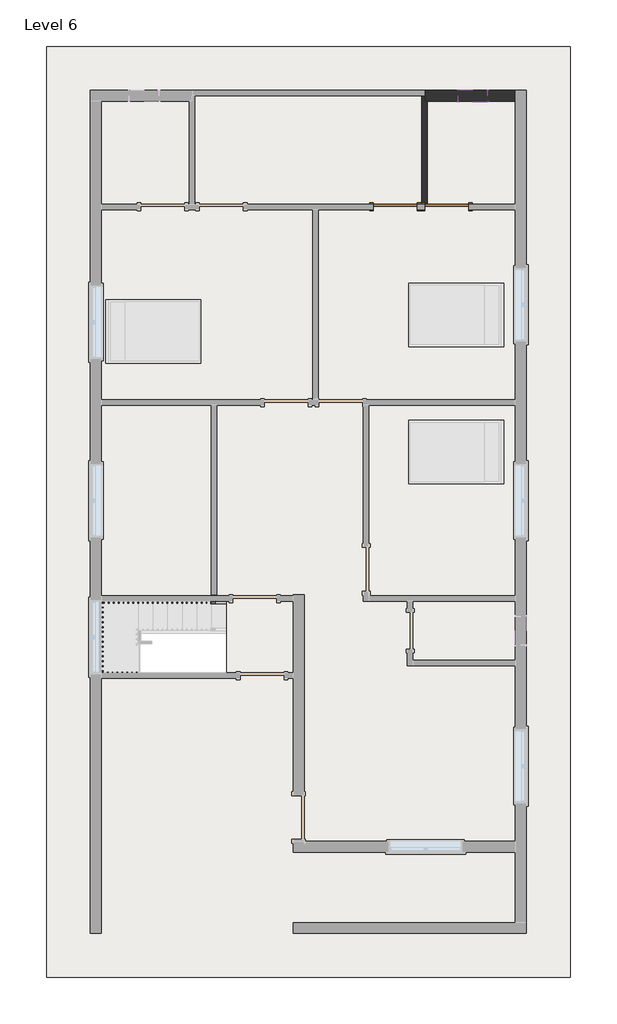
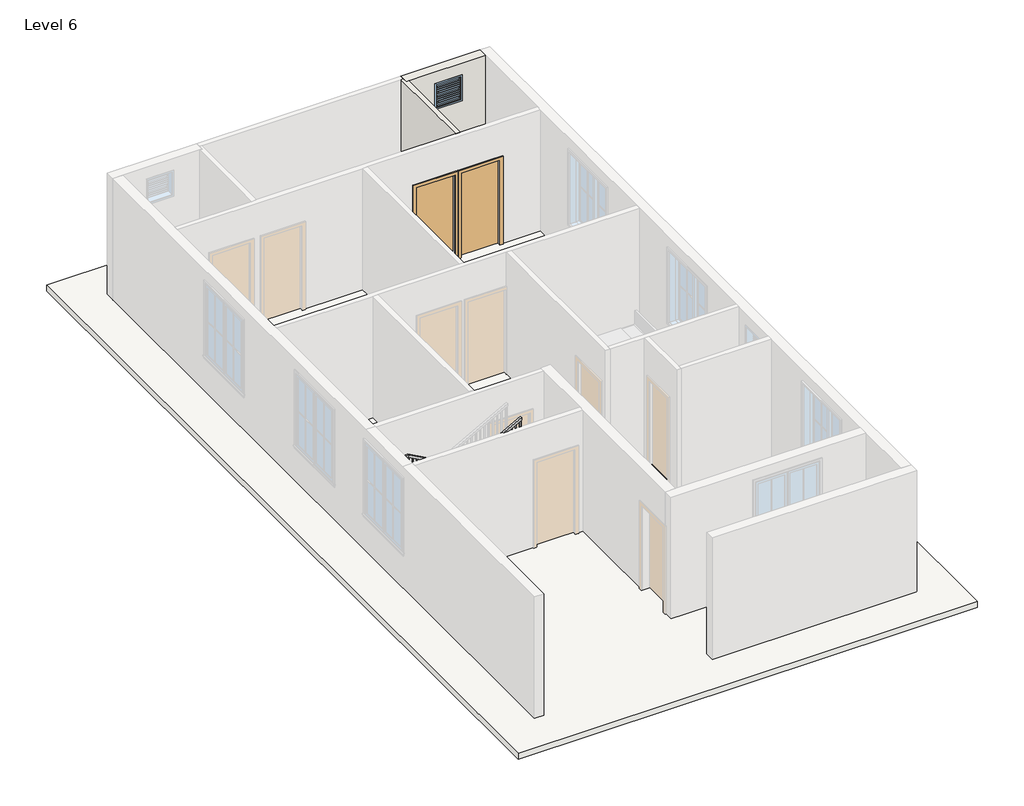
# One storey, part 2 of 3: 2 doors, 2 walls, 1 railing, 1 roof, 1 window.
"""IFC4 building model written with IfcOpenShell, lengths in millimetres."""

from ifc_helpers import new_model, si_unit, frame, origin, place, context, project, spatial, polyline, outline, extrude, faceted_brep, transform, mapped, element, save
from components import single_flush_door_3_e5f9f3c4, single_flush_door_3_305aa2a5, window_f2d8fef0

model = new_model("IFC4")

# Units and contexts
model_context = context("Model", 3, world=origin())
ifc_project = project(units=[si_unit("LENGTHUNIT", "METRE", prefix="MILLI")], contexts=[model_context])

# Site, building, storey
site = spatial("IfcSite", under=ifc_project)
building = spatial("IfcBuilding", under=site)
storey = spatial("IfcBuildingStorey", under=building, Name="Level 6", Elevation=12801.6)

# Doors
placement = place(None, origin())
single_flush_door_3_shape = single_flush_door_3_e5f9f3c4(model_context)
element("IfcDoor", 1, ObjectType="Single-Flush : DOOR 3'", at=placement, inside=storey, context=model_context, shape_type="MappedRepresentation", body=[
    mapped(single_flush_door_3_shape, transform((555.4379845, 6040.5434309, 12801.6), x_axis=(1.0, 0.0, 0.0), y_axis=(0.0, 1.0, 0.0), z_axis=(0.0, 0.0, 1.0))),
])
single_flush_door_3_2_shape = single_flush_door_3_305aa2a5(model_context)
element("IfcDoor", 2, ObjectType="Single-Flush : DOOR 3'", at=placement, inside=storey, context=model_context, shape_type="MappedRepresentation", body=[
    mapped(single_flush_door_3_2_shape, transform((1622.2379845, 6040.5434309, 12801.6), x_axis=(-1.0, 0.0, 0.0), y_axis=(0.0, -1.0, 0.0), z_axis=(0.0, 0.0, 1.0))),
])

# Railing
element("IfcRailing", 3, ObjectType="Handrail - Rectangular", at=placement, inside=storey, context=model_context, shape_type="SolidModel", body=[
    faceted_brep([(-2968.8120155, -2220.8065691, 13885.3333333), (-2968.8120155, -2220.8065691, 13827.220221), (-2968.8120155, -2170.0065691, 13827.220221), (-2968.8120155, -2170.0065691, 13885.3333333), (-4797.6120155, -2220.8065691, 14901.3333333), (-4810.7756177, -2220.8065691, 14850.5333333), (-4810.7756177, -2170.0065691, 14850.5333333), (-4797.6120155, -2170.0065691, 14901.3333333), (-5508.8120155, -2220.8065691, 14901.3333333), (-5508.8120155, -2220.8065691, 14850.5333333), (-5559.6120155, -2170.0065691, 14850.5333333), (-5559.6120155, -2170.0065691, 14901.3333333), (-5508.8120155, -3624.1565691, 14901.3333333), (-5508.8120155, -3624.1565691, 14850.5333333), (-5559.6120155, -3674.9565691, 14850.5333333), (-5559.6120155, -3674.9565691, 14901.3333333), (-5102.4120155, -3624.1565691, 14901.3333333), (-5089.2484132, -3624.1565691, 14850.5333333), (-5089.2484132, -3674.9565691, 14850.5333333), (-5102.4120155, -3674.9565691, 14901.3333333), (-2968.8120155, -3624.1565691, 16086.6666667), (-2968.8120155, -3674.9565691, 16086.6666667), (-2968.8120155, -3674.9565691, 16028.5535543), (-2968.8120155, -3624.1565691, 16028.5535543)], [[[0, 1, 2, 3]], [[1, 0, 4, 5]], [[2, 1, 5, 6]], [[3, 2, 6, 7]], [[0, 3, 7, 4]], [[5, 4, 8, 9]], [[6, 5, 9, 10]], [[7, 6, 10, 11]], [[4, 7, 11, 8]], [[9, 8, 12, 13]], [[10, 9, 13, 14]], [[11, 10, 14, 15]], [[8, 11, 15, 12]], [[13, 12, 16, 17]], [[14, 13, 17, 18]], [[15, 14, 18, 19]], [[12, 15, 19, 16]], [[20, 21, 22, 23]], [[17, 16, 20, 23]], [[18, 17, 23, 22]], [[19, 18, 22, 21]], [[16, 19, 21, 20]]]),
    extrude(outline(polyline([(16019.7341099, -2984.6870155), (16009.1507765, -3003.7370155), (15002.9333333, -3003.7370155), (15002.9333333, -2984.6870155), (16019.7341099, -2984.6870155)])), frame((0.0, -3659.0815691, 0.0), z_axis=(0.0, 1.0, 0.0), x_axis=(0.0, 0.0, 1.0)), (0.0, 0.0, 1.0), 19.05),
    extrude(outline(polyline([(15963.2896654, -3086.2870155), (15952.7063321, -3105.3370155), (15002.9333333, -3105.3370155), (15002.9333333, -3086.2870155), (15963.2896654, -3086.2870155)])), frame((0.0, -3659.0815691, 0.0), z_axis=(0.0, 1.0, 0.0), x_axis=(0.0, 0.0, 1.0)), (0.0, 0.0, 1.0), 19.05),
    extrude(outline(polyline([(15906.845221, -3187.8870155), (15896.2618876, -3206.9370155), (15002.9333333, -3206.9370155), (15002.9333333, -3187.8870155), (15906.845221, -3187.8870155)])), frame((0.0, -3659.0815691, 0.0), z_axis=(0.0, 1.0, 0.0), x_axis=(0.0, 0.0, 1.0)), (0.0, 0.0, 1.0), 19.05),
    extrude(outline(polyline([(15850.4007765, -3289.4870155), (15839.8174432, -3308.5370155), (14833.6, -3308.5370155), (14833.6, -3289.4870155), (15850.4007765, -3289.4870155)])), frame((0.0, -3659.0815691, 0.0), z_axis=(0.0, 1.0, 0.0), x_axis=(0.0, 0.0, 1.0)), (0.0, 0.0, 1.0), 19.05),
    extrude(outline(polyline([(15793.9563321, -3391.0870155), (15783.3729988, -3410.1370155), (14833.6, -3410.1370155), (14833.6, -3391.0870155), (15793.9563321, -3391.0870155)])), frame((0.0, -3659.0815691, 0.0), z_axis=(0.0, 1.0, 0.0), x_axis=(0.0, 0.0, 1.0)), (0.0, 0.0, 1.0), 19.05),
    extrude(outline(polyline([(15737.5118876, -3492.6870155), (15726.9285543, -3511.7370155), (14833.6, -3511.7370155), (14833.6, -3492.6870155), (15737.5118876, -3492.6870155)])), frame((0.0, -3659.0815691, 0.0), z_axis=(0.0, 1.0, 0.0), x_axis=(0.0, 0.0, 1.0)), (0.0, 0.0, 1.0), 19.05),
    extrude(outline(polyline([(15681.0674432, -3594.2870155), (15670.4841099, -3613.3370155), (14664.2666667, -3613.3370155), (14664.2666667, -3594.2870155), (15681.0674432, -3594.2870155)])), frame((0.0, -3659.0815691, 0.0), z_axis=(0.0, 1.0, 0.0), x_axis=(0.0, 0.0, 1.0)), (0.0, 0.0, 1.0), 19.05),
    extrude(outline(polyline([(15624.6229988, -3695.8870155), (15614.0396654, -3714.9370155), (14664.2666667, -3714.9370155), (14664.2666667, -3695.8870155), (15624.6229988, -3695.8870155)])), frame((0.0, -3659.0815691, 0.0), z_axis=(0.0, 1.0, 0.0), x_axis=(0.0, 0.0, 1.0)), (0.0, 0.0, 1.0), 19.05),
    extrude(outline(polyline([(15568.1785543, -3797.4870155), (15557.595221, -3816.5370155), (14664.2666667, -3816.5370155), (14664.2666667, -3797.4870155), (15568.1785543, -3797.4870155)])), frame((0.0, -3659.0815691, 0.0), z_axis=(0.0, 1.0, 0.0), x_axis=(0.0, 0.0, 1.0)), (0.0, 0.0, 1.0), 19.05),
    extrude(outline(polyline([(15511.7341099, -3899.0870155), (15501.1507765, -3918.1370155), (14494.9333333, -3918.1370155), (14494.9333333, -3899.0870155), (15511.7341099, -3899.0870155)])), frame((0.0, -3659.0815691, 0.0), z_axis=(0.0, 1.0, 0.0), x_axis=(0.0, 0.0, 1.0)), (0.0, 0.0, 1.0), 19.05),
    extrude(outline(polyline([(15455.2896654, -4000.6870155), (15444.7063321, -4019.7370155), (14494.9333333, -4019.7370155), (14494.9333333, -4000.6870155), (15455.2896654, -4000.6870155)])), frame((0.0, -3659.0815691, 0.0), z_axis=(0.0, 1.0, 0.0), x_axis=(0.0, 0.0, 1.0)), (0.0, 0.0, 1.0), 19.05),
    extrude(outline(polyline([(15398.845221, -4102.2870155), (15388.2618876, -4121.3370155), (14494.9333333, -4121.3370155), (14494.9333333, -4102.2870155), (15398.845221, -4102.2870155)])), frame((0.0, -3659.0815691, 0.0), z_axis=(0.0, 1.0, 0.0), x_axis=(0.0, 0.0, 1.0)), (0.0, 0.0, 1.0), 19.05),
    extrude(outline(polyline([(15342.4007765, -4203.8870155), (15331.8174432, -4222.9370155), (14325.6, -4222.9370155), (14325.6, -4203.8870155), (15342.4007765, -4203.8870155)])), frame((0.0, -3659.0815691, 0.0), z_axis=(0.0, 1.0, 0.0), x_axis=(0.0, 0.0, 1.0)), (0.0, 0.0, 1.0), 19.05),
    extrude(outline(polyline([(15285.9563321, -4305.4870155), (15275.3729988, -4324.5370155), (14325.6, -4324.5370155), (14325.6, -4305.4870155), (15285.9563321, -4305.4870155)])), frame((0.0, -3659.0815691, 0.0), z_axis=(0.0, 1.0, 0.0), x_axis=(0.0, 0.0, 1.0)), (0.0, 0.0, 1.0), 19.05),
    extrude(outline(polyline([(15229.5118876, -4407.0870155), (15218.9285543, -4426.1370155), (14325.6, -4426.1370155), (14325.6, -4407.0870155), (15229.5118876, -4407.0870155)])), frame((0.0, -3659.0815691, 0.0), z_axis=(0.0, 1.0, 0.0), x_axis=(0.0, 0.0, 1.0)), (0.0, 0.0, 1.0), 19.05),
    extrude(outline(polyline([(15173.0674432, -4508.6870155), (15162.4841099, -4527.7370155), (14156.2666667, -4527.7370155), (14156.2666667, -4508.6870155), (15173.0674432, -4508.6870155)])), frame((0.0, -3659.0815691, 0.0), z_axis=(0.0, 1.0, 0.0), x_axis=(0.0, 0.0, 1.0)), (0.0, 0.0, 1.0), 19.05),
    extrude(outline(polyline([(15116.6229988, -4610.2870155), (15106.0396654, -4629.3370155), (14156.2666667, -4629.3370155), (14156.2666667, -4610.2870155), (15116.6229988, -4610.2870155)])), frame((0.0, -3659.0815691, 0.0), z_axis=(0.0, 1.0, 0.0), x_axis=(0.0, 0.0, 1.0)), (0.0, 0.0, 1.0), 19.05),
    extrude(outline(polyline([(15060.1785543, -4711.8870155), (15049.595221, -4730.9370155), (14156.2666667, -4730.9370155), (14156.2666667, -4711.8870155), (15060.1785543, -4711.8870155)])), frame((0.0, -3659.0815691, 0.0), z_axis=(0.0, 1.0, 0.0), x_axis=(0.0, 0.0, 1.0)), (0.0, 0.0, 1.0), 19.05),
    extrude(outline(polyline([(15003.7341099, -4813.4870155), (14993.1507765, -4832.5370155), (13986.9333333, -4832.5370155), (13986.9333333, -4813.4870155), (15003.7341099, -4813.4870155)])), frame((0.0, -3659.0815691, 0.0), z_axis=(0.0, 1.0, 0.0), x_axis=(0.0, 0.0, 1.0)), (0.0, 0.0, 1.0), 19.05),
    extrude(outline(polyline([(14947.2896654, -4915.0870155), (14936.7063321, -4934.1370155), (13986.9333333, -4934.1370155), (13986.9333333, -4915.0870155), (14947.2896654, -4915.0870155)])), frame((0.0, -3659.0815691, 0.0), z_axis=(0.0, 1.0, 0.0), x_axis=(0.0, 0.0, 1.0)), (0.0, 0.0, 1.0), 19.05),
    extrude(outline(polyline([(14890.845221, -5016.6870155), (14880.2618876, -5035.7370155), (13986.9333333, -5035.7370155), (13986.9333333, -5016.6870155), (14890.845221, -5016.6870155)])), frame((0.0, -3659.0815691, 0.0), z_axis=(0.0, 1.0, 0.0), x_axis=(0.0, 0.0, 1.0)), (0.0, 0.0, 1.0), 19.05),
    extrude(outline(polyline([(-5137.3370155, -3659.0815691), (-5137.3370155, -3640.0315691), (-5118.2870155, -3640.0315691), (-5118.2870155, -3659.0815691), (-5137.3370155, -3659.0815691)])), frame((0.0, 0.0, 13986.9333333), z_axis=(0.0, 0.0, 1.0), x_axis=(1.0, 0.0, 0.0)), (0.0, 0.0, 1.0), 863.6),
    extrude(outline(polyline([(-5238.9370155, -3659.0815691), (-5238.9370155, -3640.0315691), (-5219.8870155, -3640.0315691), (-5219.8870155, -3659.0815691), (-5238.9370155, -3659.0815691)])), frame((0.0, 0.0, 13986.9333333), z_axis=(0.0, 0.0, 1.0), x_axis=(1.0, 0.0, 0.0)), (0.0, 0.0, 1.0), 863.6),
    extrude(outline(polyline([(-5340.5370155, -3659.0815691), (-5340.5370155, -3640.0315691), (-5321.4870155, -3640.0315691), (-5321.4870155, -3659.0815691), (-5340.5370155, -3659.0815691)])), frame((0.0, 0.0, 13986.9333333), z_axis=(0.0, 0.0, 1.0), x_axis=(1.0, 0.0, 0.0)), (0.0, 0.0, 1.0), 863.6),
    extrude(outline(polyline([(-5442.1370155, -3659.0815691), (-5442.1370155, -3640.0315691), (-5423.0870155, -3640.0315691), (-5423.0870155, -3659.0815691), (-5442.1370155, -3659.0815691)])), frame((0.0, 0.0, 13986.9333333), z_axis=(0.0, 0.0, 1.0), x_axis=(1.0, 0.0, 0.0)), (0.0, 0.0, 1.0), 863.6),
    extrude(outline(polyline([(-5543.7370155, -3608.2815691), (-5524.6870155, -3608.2815691), (-5524.6870155, -3627.3315691), (-5543.7370155, -3627.3315691), (-5543.7370155, -3608.2815691)])), frame((0.0, 0.0, 13986.9333333), z_axis=(0.0, 0.0, 1.0), x_axis=(1.0, 0.0, 0.0)), (0.0, 0.0, 1.0), 863.6),
    extrude(outline(polyline([(-5543.7370155, -3506.6815691), (-5524.6870155, -3506.6815691), (-5524.6870155, -3525.7315691), (-5543.7370155, -3525.7315691), (-5543.7370155, -3506.6815691)])), frame((0.0, 0.0, 13986.9333333), z_axis=(0.0, 0.0, 1.0), x_axis=(1.0, 0.0, 0.0)), (0.0, 0.0, 1.0), 863.6),
    extrude(outline(polyline([(-5543.7370155, -3405.0815691), (-5524.6870155, -3405.0815691), (-5524.6870155, -3424.1315691), (-5543.7370155, -3424.1315691), (-5543.7370155, -3405.0815691)])), frame((0.0, 0.0, 13986.9333333), z_axis=(0.0, 0.0, 1.0), x_axis=(1.0, 0.0, 0.0)), (0.0, 0.0, 1.0), 863.6),
    extrude(outline(polyline([(-5543.7370155, -3303.4815691), (-5524.6870155, -3303.4815691), (-5524.6870155, -3322.5315691), (-5543.7370155, -3322.5315691), (-5543.7370155, -3303.4815691)])), frame((0.0, 0.0, 13986.9333333), z_axis=(0.0, 0.0, 1.0), x_axis=(1.0, 0.0, 0.0)), (0.0, 0.0, 1.0), 863.6),
    extrude(outline(polyline([(-5543.7370155, -3201.8815691), (-5524.6870155, -3201.8815691), (-5524.6870155, -3220.9315691), (-5543.7370155, -3220.9315691), (-5543.7370155, -3201.8815691)])), frame((0.0, 0.0, 13986.9333333), z_axis=(0.0, 0.0, 1.0), x_axis=(1.0, 0.0, 0.0)), (0.0, 0.0, 1.0), 863.6),
    extrude(outline(polyline([(-5543.7370155, -3100.2815691), (-5524.6870155, -3100.2815691), (-5524.6870155, -3119.3315691), (-5543.7370155, -3119.3315691), (-5543.7370155, -3100.2815691)])), frame((0.0, 0.0, 13986.9333333), z_axis=(0.0, 0.0, 1.0), x_axis=(1.0, 0.0, 0.0)), (0.0, 0.0, 1.0), 863.6),
    extrude(outline(polyline([(-5543.7370155, -2998.6815691), (-5524.6870155, -2998.6815691), (-5524.6870155, -3017.7315691), (-5543.7370155, -3017.7315691), (-5543.7370155, -2998.6815691)])), frame((0.0, 0.0, 13986.9333333), z_axis=(0.0, 0.0, 1.0), x_axis=(1.0, 0.0, 0.0)), (0.0, 0.0, 1.0), 863.6),
    extrude(outline(polyline([(-5543.7370155, -2897.0815691), (-5524.6870155, -2897.0815691), (-5524.6870155, -2916.1315691), (-5543.7370155, -2916.1315691), (-5543.7370155, -2897.0815691)])), frame((0.0, 0.0, 13986.9333333), z_axis=(0.0, 0.0, 1.0), x_axis=(1.0, 0.0, 0.0)), (0.0, 0.0, 1.0), 863.6),
    extrude(outline(polyline([(-5543.7370155, -2795.4815691), (-5524.6870155, -2795.4815691), (-5524.6870155, -2814.5315691), (-5543.7370155, -2814.5315691), (-5543.7370155, -2795.4815691)])), frame((0.0, 0.0, 13986.9333333), z_axis=(0.0, 0.0, 1.0), x_axis=(1.0, 0.0, 0.0)), (0.0, 0.0, 1.0), 863.6),
    extrude(outline(polyline([(-5543.7370155, -2693.8815691), (-5524.6870155, -2693.8815691), (-5524.6870155, -2712.9315691), (-5543.7370155, -2712.9315691), (-5543.7370155, -2693.8815691)])), frame((0.0, 0.0, 13986.9333333), z_axis=(0.0, 0.0, 1.0), x_axis=(1.0, 0.0, 0.0)), (0.0, 0.0, 1.0), 863.6),
    extrude(outline(polyline([(-5543.7370155, -2592.2815691), (-5524.6870155, -2592.2815691), (-5524.6870155, -2611.3315691), (-5543.7370155, -2611.3315691), (-5543.7370155, -2592.2815691)])), frame((0.0, 0.0, 13986.9333333), z_axis=(0.0, 0.0, 1.0), x_axis=(1.0, 0.0, 0.0)), (0.0, 0.0, 1.0), 863.6),
    extrude(outline(polyline([(-5543.7370155, -2490.6815691), (-5524.6870155, -2490.6815691), (-5524.6870155, -2509.7315691), (-5543.7370155, -2509.7315691), (-5543.7370155, -2490.6815691)])), frame((0.0, 0.0, 13986.9333333), z_axis=(0.0, 0.0, 1.0), x_axis=(1.0, 0.0, 0.0)), (0.0, 0.0, 1.0), 863.6),
    extrude(outline(polyline([(-5543.7370155, -2389.0815691), (-5524.6870155, -2389.0815691), (-5524.6870155, -2408.1315691), (-5543.7370155, -2408.1315691), (-5543.7370155, -2389.0815691)])), frame((0.0, 0.0, 13986.9333333), z_axis=(0.0, 0.0, 1.0), x_axis=(1.0, 0.0, 0.0)), (0.0, 0.0, 1.0), 863.6),
    extrude(outline(polyline([(-5543.7370155, -2287.4815691), (-5524.6870155, -2287.4815691), (-5524.6870155, -2306.5315691), (-5543.7370155, -2306.5315691), (-5543.7370155, -2287.4815691)])), frame((0.0, 0.0, 13986.9333333), z_axis=(0.0, 0.0, 1.0), x_axis=(1.0, 0.0, 0.0)), (0.0, 0.0, 1.0), 863.6),
    extrude(outline(polyline([(-5499.2870155, -2185.8815691), (-5499.2870155, -2204.9315691), (-5518.3370155, -2204.9315691), (-5518.3370155, -2185.8815691), (-5499.2870155, -2185.8815691)])), frame((0.0, 0.0, 13986.9333333), z_axis=(0.0, 0.0, 1.0), x_axis=(1.0, 0.0, 0.0)), (0.0, 0.0, 1.0), 863.6),
    extrude(outline(polyline([(-5397.6870155, -2185.8815691), (-5397.6870155, -2204.9315691), (-5416.7370155, -2204.9315691), (-5416.7370155, -2185.8815691), (-5397.6870155, -2185.8815691)])), frame((0.0, 0.0, 13986.9333333), z_axis=(0.0, 0.0, 1.0), x_axis=(1.0, 0.0, 0.0)), (0.0, 0.0, 1.0), 863.6),
    extrude(outline(polyline([(-5296.0870155, -2185.8815691), (-5296.0870155, -2204.9315691), (-5315.1370155, -2204.9315691), (-5315.1370155, -2185.8815691), (-5296.0870155, -2185.8815691)])), frame((0.0, 0.0, 13986.9333333), z_axis=(0.0, 0.0, 1.0), x_axis=(1.0, 0.0, 0.0)), (0.0, 0.0, 1.0), 863.6),
    extrude(outline(polyline([(-5194.4870155, -2185.8815691), (-5194.4870155, -2204.9315691), (-5213.5370155, -2204.9315691), (-5213.5370155, -2185.8815691), (-5194.4870155, -2185.8815691)])), frame((0.0, 0.0, 13986.9333333), z_axis=(0.0, 0.0, 1.0), x_axis=(1.0, 0.0, 0.0)), (0.0, 0.0, 1.0), 863.6),
    extrude(outline(polyline([(-5092.8870155, -2185.8815691), (-5092.8870155, -2204.9315691), (-5111.9370155, -2204.9315691), (-5111.9370155, -2185.8815691), (-5092.8870155, -2185.8815691)])), frame((0.0, 0.0, 13986.9333333), z_axis=(0.0, 0.0, 1.0), x_axis=(1.0, 0.0, 0.0)), (0.0, 0.0, 1.0), 863.6),
    extrude(outline(polyline([(-4991.2870155, -2185.8815691), (-4991.2870155, -2204.9315691), (-5010.3370155, -2204.9315691), (-5010.3370155, -2185.8815691), (-4991.2870155, -2185.8815691)])), frame((0.0, 0.0, 13986.9333333), z_axis=(0.0, 0.0, 1.0), x_axis=(1.0, 0.0, 0.0)), (0.0, 0.0, 1.0), 863.6),
    extrude(outline(polyline([(-4889.6870155, -2185.8815691), (-4889.6870155, -2204.9315691), (-4908.7370155, -2204.9315691), (-4908.7370155, -2185.8815691), (-4889.6870155, -2185.8815691)])), frame((0.0, 0.0, 13986.9333333), z_axis=(0.0, 0.0, 1.0), x_axis=(1.0, 0.0, 0.0)), (0.0, 0.0, 1.0), 863.6),
    extrude(outline(polyline([(14837.9285543, -4788.0870155), (14848.5118876, -4807.1370155), (13986.9333333, -4807.1370155), (13986.9333333, -4788.0870155), (14837.9285543, -4788.0870155)])), frame((0.0, -2204.9315691, 0.0), z_axis=(0.0, 1.0, 0.0), x_axis=(0.0, 0.0, 1.0)), (0.0, 0.0, 1.0), 19.05),
    extrude(outline(polyline([(14781.4841099, -4686.4870155), (14792.0674432, -4705.5370155), (13817.6, -4705.5370155), (13817.6, -4686.4870155), (14781.4841099, -4686.4870155)])), frame((0.0, -2204.9315691, 0.0), z_axis=(0.0, 1.0, 0.0), x_axis=(0.0, 0.0, 1.0)), (0.0, 0.0, 1.0), 19.05),
    extrude(outline(polyline([(14725.0396654, -4584.8870155), (14735.6229988, -4603.9370155), (13817.6, -4603.9370155), (13817.6, -4584.8870155), (14725.0396654, -4584.8870155)])), frame((0.0, -2204.9315691, 0.0), z_axis=(0.0, 1.0, 0.0), x_axis=(0.0, 0.0, 1.0)), (0.0, 0.0, 1.0), 19.05),
    extrude(outline(polyline([(14668.595221, -4483.2870155), (14679.1785543, -4502.3370155), (13817.6, -4502.3370155), (13817.6, -4483.2870155), (14668.595221, -4483.2870155)])), frame((0.0, -2204.9315691, 0.0), z_axis=(0.0, 1.0, 0.0), x_axis=(0.0, 0.0, 1.0)), (0.0, 0.0, 1.0), 19.05),
    extrude(outline(polyline([(14612.1507765, -4381.6870155), (14622.7341099, -4400.7370155), (13648.2666667, -4400.7370155), (13648.2666667, -4381.6870155), (14612.1507765, -4381.6870155)])), frame((0.0, -2204.9315691, 0.0), z_axis=(0.0, 1.0, 0.0), x_axis=(0.0, 0.0, 1.0)), (0.0, 0.0, 1.0), 19.05),
    extrude(outline(polyline([(14555.7063321, -4280.0870155), (14566.2896654, -4299.1370155), (13648.2666667, -4299.1370155), (13648.2666667, -4280.0870155), (14555.7063321, -4280.0870155)])), frame((0.0, -2204.9315691, 0.0), z_axis=(0.0, 1.0, 0.0), x_axis=(0.0, 0.0, 1.0)), (0.0, 0.0, 1.0), 19.05),
    extrude(outline(polyline([(14499.2618876, -4178.4870155), (14509.845221, -4197.5370155), (13648.2666667, -4197.5370155), (13648.2666667, -4178.4870155), (14499.2618876, -4178.4870155)])), frame((0.0, -2204.9315691, 0.0), z_axis=(0.0, 1.0, 0.0), x_axis=(0.0, 0.0, 1.0)), (0.0, 0.0, 1.0), 19.05),
    extrude(outline(polyline([(14442.8174432, -4076.8870155), (14453.4007765, -4095.9370155), (13478.9333333, -4095.9370155), (13478.9333333, -4076.8870155), (14442.8174432, -4076.8870155)])), frame((0.0, -2204.9315691, 0.0), z_axis=(0.0, 1.0, 0.0), x_axis=(0.0, 0.0, 1.0)), (0.0, 0.0, 1.0), 19.05),
    extrude(outline(polyline([(14386.3729988, -3975.2870155), (14396.9563321, -3994.3370155), (13478.9333333, -3994.3370155), (13478.9333333, -3975.2870155), (14386.3729988, -3975.2870155)])), frame((0.0, -2204.9315691, 0.0), z_axis=(0.0, 1.0, 0.0), x_axis=(0.0, 0.0, 1.0)), (0.0, 0.0, 1.0), 19.05),
    extrude(outline(polyline([(14329.9285543, -3873.6870155), (14340.5118876, -3892.7370155), (13478.9333333, -3892.7370155), (13478.9333333, -3873.6870155), (14329.9285543, -3873.6870155)])), frame((0.0, -2204.9315691, 0.0), z_axis=(0.0, 1.0, 0.0), x_axis=(0.0, 0.0, 1.0)), (0.0, 0.0, 1.0), 19.05),
    extrude(outline(polyline([(14273.4841099, -3772.0870155), (14284.0674432, -3791.1370155), (13309.6, -3791.1370155), (13309.6, -3772.0870155), (14273.4841099, -3772.0870155)])), frame((0.0, -2204.9315691, 0.0), z_axis=(0.0, 1.0, 0.0), x_axis=(0.0, 0.0, 1.0)), (0.0, 0.0, 1.0), 19.05),
    extrude(outline(polyline([(14217.0396654, -3670.4870155), (14227.6229988, -3689.5370155), (13309.6, -3689.5370155), (13309.6, -3670.4870155), (14217.0396654, -3670.4870155)])), frame((0.0, -2204.9315691, 0.0), z_axis=(0.0, 1.0, 0.0), x_axis=(0.0, 0.0, 1.0)), (0.0, 0.0, 1.0), 19.05),
    extrude(outline(polyline([(14160.595221, -3568.8870155), (14171.1785543, -3587.9370155), (13309.6, -3587.9370155), (13309.6, -3568.8870155), (14160.595221, -3568.8870155)])), frame((0.0, -2204.9315691, 0.0), z_axis=(0.0, 1.0, 0.0), x_axis=(0.0, 0.0, 1.0)), (0.0, 0.0, 1.0), 19.05),
    extrude(outline(polyline([(14104.1507765, -3467.2870155), (14114.7341099, -3486.3370155), (13140.2666667, -3486.3370155), (13140.2666667, -3467.2870155), (14104.1507765, -3467.2870155)])), frame((0.0, -2204.9315691, 0.0), z_axis=(0.0, 1.0, 0.0), x_axis=(0.0, 0.0, 1.0)), (0.0, 0.0, 1.0), 19.05),
    extrude(outline(polyline([(14047.7063321, -3365.6870155), (14058.2896654, -3384.7370155), (13140.2666667, -3384.7370155), (13140.2666667, -3365.6870155), (14047.7063321, -3365.6870155)])), frame((0.0, -2204.9315691, 0.0), z_axis=(0.0, 1.0, 0.0), x_axis=(0.0, 0.0, 1.0)), (0.0, 0.0, 1.0), 19.05),
    extrude(outline(polyline([(13991.2618876, -3264.0870155), (14001.845221, -3283.1370155), (13140.2666667, -3283.1370155), (13140.2666667, -3264.0870155), (13991.2618876, -3264.0870155)])), frame((0.0, -2204.9315691, 0.0), z_axis=(0.0, 1.0, 0.0), x_axis=(0.0, 0.0, 1.0)), (0.0, 0.0, 1.0), 19.05),
    extrude(outline(polyline([(13934.8174432, -3162.4870155), (13945.4007765, -3181.5370155), (12970.9333333, -3181.5370155), (12970.9333333, -3162.4870155), (13934.8174432, -3162.4870155)])), frame((0.0, -2204.9315691, 0.0), z_axis=(0.0, 1.0, 0.0), x_axis=(0.0, 0.0, 1.0)), (0.0, 0.0, 1.0), 19.05),
    extrude(outline(polyline([(13878.3729988, -3060.8870155), (13888.9563321, -3079.9370155), (12970.9333333, -3079.9370155), (12970.9333333, -3060.8870155), (13878.3729988, -3060.8870155)])), frame((0.0, -2204.9315691, 0.0), z_axis=(0.0, 1.0, 0.0), x_axis=(0.0, 0.0, 1.0)), (0.0, 0.0, 1.0), 19.05),
    extrude(outline(polyline([(-5543.7370155, -3640.0315691), (-5524.6870155, -3640.0315691), (-5524.6870155, -3659.0815691), (-5543.7370155, -3659.0815691), (-5543.7370155, -3640.0315691)])), frame((0.0, 0.0, 13986.9333333), z_axis=(0.0, 0.0, 1.0), x_axis=(1.0, 0.0, 0.0)), (0.0, 0.0, 1.0), 863.6),
    extrude(outline(polyline([(-5524.6870155, -2185.8815691), (-5524.6870155, -2204.9315691), (-5543.7370155, -2204.9315691), (-5543.7370155, -2185.8815691), (-5524.6870155, -2185.8815691)])), frame((0.0, 0.0, 13986.9333333), z_axis=(0.0, 0.0, 1.0), x_axis=(1.0, 0.0, 0.0)), (0.0, 0.0, 1.0), 863.6),
    extrude(outline(polyline([(16028.5535543, -2968.8120155), (16017.970221, -2987.8620155), (15002.9333333, -2987.8620155), (15002.9333333, -2968.8120155), (16028.5535543, -2968.8120155)])), frame((0.0, -3659.0815691, 0.0), z_axis=(0.0, 1.0, 0.0), x_axis=(0.0, 0.0, 1.0)), (0.0, 0.0, 1.0), 19.05),
    extrude(outline(polyline([(13827.220221, -2968.8120155), (13837.8035543, -2987.8620155), (12970.9333333, -2987.8620155), (12970.9333333, -2968.8120155), (13827.220221, -2968.8120155)])), frame((0.0, -2204.9315691, 0.0), z_axis=(0.0, 1.0, 0.0), x_axis=(0.0, 0.0, 1.0)), (0.0, 0.0, 1.0), 19.05),
])

# Roof
element("IfcRoof", 4, ObjectType="ROOF 6\"", at=placement, inside=storey, context=model_context, shape_type="SweptSolid", body=[
    extrude(outline(polyline([(4193.9879845, 9374.2934309), (4193.9879845, -9993.2065691), (-6702.6120155, -9993.2065691), (-6702.6120155, 9374.2934309), (4193.9879845, 9374.2934309)]), holes=[polyline([(-2968.8120155, -2150.9565691), (-5788.2120155, -2150.9565691), (-5788.2120155, -3674.9565691), (-2968.8120155, -3674.9565691), (-2968.8120155, -2150.9565691)])]), frame((0.0, 0.0, 12649.2), z_axis=(0.0, 0.0, 1.0), x_axis=(1.0, 0.0, 0.0)), (0.0, 0.0, 1.0), 152.4),
])

# Walls
element("IfcWall", 5, ObjectType="WALL 4.5\"", at=placement, inside=storey, context=model_context, shape_type="SweptSolid", body=[
    extrude(outline(polyline([(1107.8879845, 6097.6934309), (1107.8879845, 8345.5934309), (1165.0379845, 8345.5934309), (1165.0379845, 8231.2934309), (1222.1879845, 8231.2934309), (1222.1879845, 6097.6934309), (1107.8879845, 6097.6934309)])), frame((0.0, 0.0, 12801.6), z_axis=(0.0, 0.0, 1.0), x_axis=(1.0, 0.0, 0.0)), (0.0, 0.0, 1.0), 3048.0),
])
element("IfcWall", 6, ObjectType="WALL 9\"", at=placement, inside=storey, context=model_context, shape_type="Brep", body=[
    faceted_brep([(3050.9879845, 8459.8934309, 12801.6), (1165.0379845, 8459.8934309, 12801.6), (1165.0379845, 8459.8934309, 15849.6), (3050.9879845, 8459.8934309, 15849.6), (2469.9629845, 8459.8934309, 15544.8), (1860.3629845, 8459.8934309, 15544.8), (1860.3629845, 8459.8934309, 14935.2), (2469.9629845, 8459.8934309, 14935.2), (3050.9879845, 8231.2934309, 12801.6), (3050.9879845, 8231.2934309, 15849.6), (1222.1879845, 8231.2934309, 15849.6), (1165.0379845, 8231.2934309, 15849.6), (1165.0379845, 8231.2934309, 12801.6), (1222.1879845, 8231.2934309, 12801.6), (2469.9629845, 8231.2934309, 15544.8), (2469.9629845, 8231.2934309, 14935.2), (1860.3629845, 8231.2934309, 14935.2), (1860.3629845, 8231.2934309, 15544.8), (1165.0379845, 8345.5934309, 12801.6), (1165.0379845, 8345.5934309, 15849.6)], [[[0, 1, 2, 3], [4, 5, 6, 7]], [[8, 9, 10, 11, 12, 13], [14, 15, 16, 17]], [[1, 0, 8, 13, 12, 18]], [[2, 1, 18, 12, 11, 19]], [[0, 3, 9, 8]], [[15, 14, 4, 7]], [[16, 15, 7, 6]], [[17, 16, 6, 5]], [[14, 17, 5, 4]], [[3, 2, 19, 11, 10, 9]]]),
])

# Window
window_shape = window_f2d8fef0(model_context)
element("IfcWindow", 7, ObjectType="Window-Louvers : 24\" x 24\"", at=placement, inside=storey, context=model_context, shape_type="MappedRepresentation", body=[
    mapped(window_shape, transform((2165.1629845, 8339.2434309, 14020.8), x_axis=(-1.0, 0.0, 0.0), y_axis=(0.0, -1.0, 0.0), z_axis=(0.0, 0.0, 1.0))),
])

save(model, "model.ifc")

# Revit data of these elements
# Type "Single-Flush : DOOR 3'"
#   Type Mark = "9"
#   Construction Type Id = "MDOOR"
#   Assembly Code = "C1020"
#   Analytic Construction = "Metal"
#   Thickness = 0' - 2"
#   Heat Transfer Coefficient (U) = 0.651978 BTU/(h·ft²·°F)
#   Height = 7' - 0"
#   Trim Projection Ext = 0' - 1"
#   Trim Projection Int = 0' - 1"
#   Trim Width = 0' - 3"
#   Width = 3' - 0"
#   Define Thermal Properties by = 1
#   Door Material = Door - Panel
#   Frame Material = Door - Frame
#   Visual Light Transmittance = 0
#   Solar Heat Gain Coefficient = 0
#   Function = (empty or 0)
#   Wall Closure = (empty or 0)
# Type "Handrail - Rectangular"
#   Assembly Code = "C2010400"
#   built-in parameter 1008612 = 0.0416667 (stored number, unit not read)
#   built-in parameter 1008611 = 0.0416667 (stored number, unit not read)
#   built-in parameter 1008609 = 0.333333 (stored number, unit not read)
#   built-in parameter 1008604 = 0.166667 (stored number, unit not read)
#   built-in parameter 1008603 = 0.166667 (stored number, unit not read)
#   Railing Height = 3' - 0"
#   built-in parameter 1008630 = 2
#   built-in parameter 1008610 = 2
#   built-in parameter 1008618 = Baluster - Square : 3/4"
# Type "ROOF 6\""
#   Assembly Code = "B1020"
#   Layers, outside or top first: 0' - 6" no material (function 1)
# Type "WALL 4.5\""
#   Assembly Code = "B2010"
#   Layers, outside or top first: 0' - 4 1/2" no material (function 1)
# Type "WALL 9\""
#   Assembly Code = "B2010"
#   Layers, outside or top first: 0' - 9" no material (function 1)
# Type "Window-Louvers : 24\" x 24\""
#   Type Mark = "19"
#   Construction Type Id = "GSP4R"
#   Assembly Code = "B20"
#   Analytic Construction = "1/8 in Pilkington single glazing"
#   Visual Light Transmittance = 0.9
#   Thermal Resistance (R) = 1.53941 (h·ft²·°F)/BTU
#   Solar Heat Gain Coefficient = 0.78
#   Max Height = 1' - 11.74264"
#   Height = 2' - 0"
#   Heat Transfer Coefficient (U) = 0.6496 BTU/(h·ft²·°F)
#   Blade Width [instance default] = 1' - 10 1/2"
#   Blade Vertical Thickness = 0' - 0.35355"
#   Blade Thickness = 0' - 0 1/4"
#   Blade Spacing = 0' - 1 1/2"
#   Blade Height = 0' - 1.85355"
#   Blade Depth = 0' - 3"
#   Blade Angle = 45.00°
#   Default Sill Height = 3' - 0"
#   Trim Projection_Exterior = 0' - 0 1/2"
#   Trim Projection_Interior = 0' - 0 1/2"
#   Trim Width_Exterior = 0' - 1 1/2"
#   Trim Width_Interior = 0' - 1 1/2"
#   Width = 2' - 0"
#   Max Blade Count = 12
#   Define Thermal Properties by = 1
#   Blade Count = 12
#   Frame Material = Birch
#   Louver Material = Birch
#   Trim Exterior Material = Birch
#   Trim Interior Material = Birch
#   Wall Closure = (empty or 0)
# Elements 1, 2 (IfcDoor, "Single-Flush : DOOR 3'")
#   Phase Created = New Construction
#   Materials on its faces: "Door - Frame", "Door - Panel"
# Element 3 (IfcRailing, "Handrail - Rectangular")
#   Phase Created = New Construction
# Element 4 (IfcRoof, "ROOF 6\"")
#   built-in parameter 1001705 = 42 (stored number, unit not read)
#   built-in parameter 1001701 = -0.5 (stored number, unit not read)
#   built-in parameter 1001710 = 33615
#   Phase Created = New Construction
#   Materials on its faces: "Default Roof", "Brick, Common", "Birch"
# Element 5 (IfcWall, "WALL 4.5\"")
#   Top Offset = 0' - 0"
#   Base Offset = 0' - 0"
#   Unconnected Height = 10' - 0"
#   wall height = 10' - 0"
#   Phase Created = New Construction
#   Base Constraint = Level 6
#   Materials on its faces: "Default Wall"
# Element 6 (IfcWall, "WALL 9\"")
#   Top Offset = 0' - 0"
#   Base Offset = 0' - 0"
#   Unconnected Height = 10' - 0"
#   wall height = 10' - 0"
#   Phase Created = New Construction
#   Base Constraint = Level 6
#   Materials on its faces: "Default Wall", "Brick, Common"
# Element 7 (IfcWindow, "Window-Louvers : 24\" x 24\"")
#   Mark = "49"
#   Blade Width = 1' - 10 1/2"
#   Phase Created = New Construction
#   Materials on its faces: "Birch"
# Materials
#   "Door - Panel": class "Wood", colour RGB 210 159 95, transparency 0, Cost = 0
#   "Door - Frame": colour RGB 118 70 51, transparency 0, Cost = 0
#   "Birch": class "Wood", colour RGB 224 178 126, transparency 0, Description = "Betula Alleghaniensis", Cost = 0
#   "Default Roof": colour RGB 88 101 114, transparency 0, Cost = 0
#   "Brick, Common": class "Masonry", colour RGB 170 98 104, transparency 0, Description = "Common brick", Cost = 0
#   "Default Wall": colour RGB 128 128 128, transparency 0, Cost = 0
